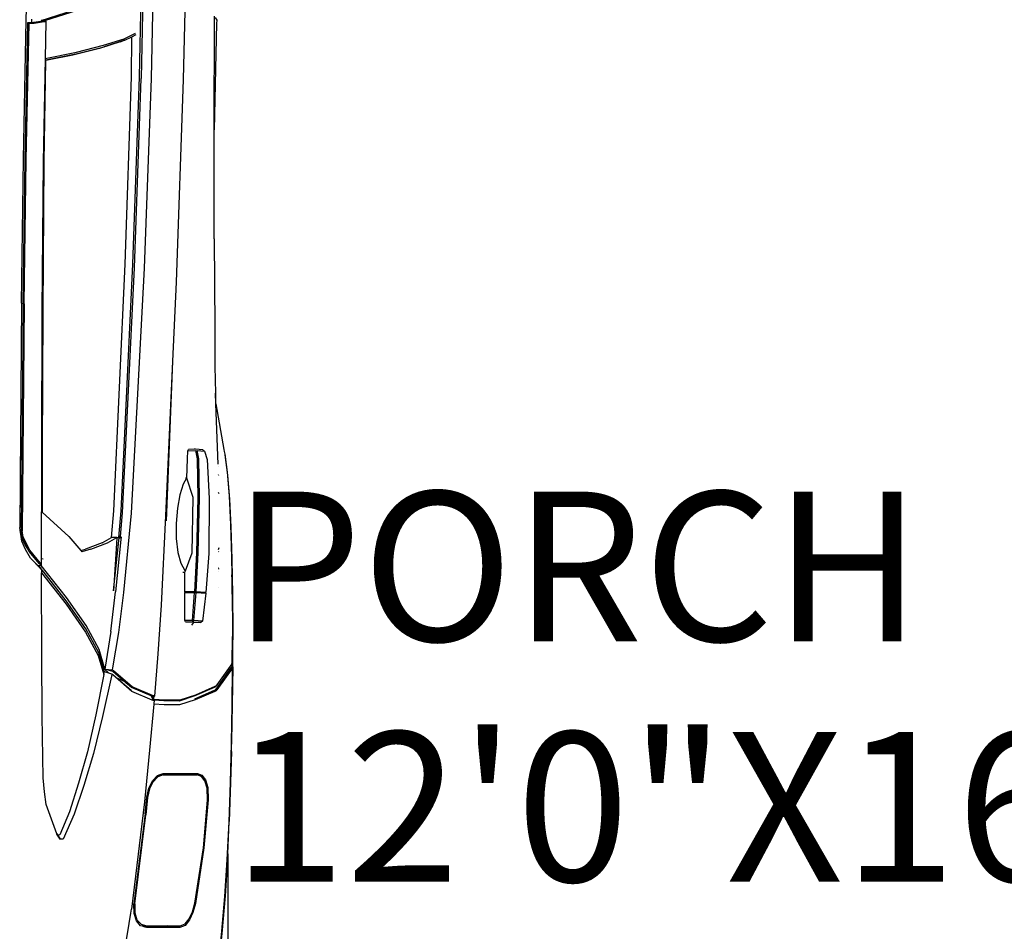
# Model space of a CAD drawing. Units: inches. Extents: x 22042254 to 25404563, y 17568978 to 17626777.
# Tile 30 of 45: x 22179876 to 22179932, y 17626227 to 17626279. Entities that reach past the tile are written whole.
import ezdxf

# ---------------------------------------------------------------- set-up
doc = ezdxf.new("R2010")
doc.units = ezdxf.units.IN
doc.header["$MEASUREMENT"] = 0
doc.layers.add('A-AREA-IDEN', color=7, linetype='Continuous', lineweight=18)
doc.layers.add('A-SITE-VEHI', color=8, linetype='Continuous', lineweight=18)
doc.layers.add('Edges', color=250, linetype='Continuous')
doc.styles.get("Standard").update_dxf_attribs({"font": 'arial.ttf'})

# ---------------------------------------------------------------- blocks, each defined once
blk = doc.blocks.new('Nissan Qashqai pl')
at = {"layer": 'Edges'}
for p, q in [((10.4304, 12.8056), (10.4339, 12.8061)), ((10.4339, 12.8061), (10.4573, 12.8093)), ((10.4339, 12.8061), (10.4345, 12.8062)), ((10.4345, 12.8062), (10.4613, 12.8099)), ((10.4573, 12.8093), (10.4889, 12.8119)), ((10.4613, 12.8099), (10.4926, 12.8125)), ((10.4889, 12.8119), (10.526, 12.8138)), ((10.4926, 12.8125), (10.5294, 12.8143)), ((10.526, 12.8138), (10.569, 12.8151)), ((10.5294, 12.8143), (10.5719, 12.8156)), ((10.569, 12.8151), (10.5919, 12.8155)), ((10.5719, 12.8156), (10.6176, 12.8164)), ((10.5919, 12.8155), (10.6151, 12.8159)), ((10.5981, 12.8157), (10.5919, 12.8155)), ((10.6174, 12.816), (10.5981, 12.8157)), ((10.6151, 12.8159), (10.6644, 12.8162)), ((10.6176, 12.8164), (10.6651, 12.8167)), ((10.6644, 12.8162), (10.7078, 12.8159)), ((10.6651, 12.8167), (10.666, 12.8167)), ((10.666, 12.8167), (10.677, 12.8167)), ((10.6729, 12.8157), (10.7082, 12.8156)), ((10.6809, 12.8167), (10.677, 12.8167)), ((10.7128, 12.8166), (10.6809, 12.8167)), ((10.7078, 12.8159), (10.7083, 12.8156)), ((10.7082, 12.8156), (10.7078, 12.8159)), ((10.7085, 12.8153), (10.7082, 12.8156)), ((10.7082, 12.8156), (10.7083, 12.8156)), ((10.7083, 12.8156), (10.7087, 12.8153)), ((10.7083, 12.8156), (10.7125, 12.8156)), ((10.7087, 12.8153), (10.7363, 12.7959)), ((10.7139, 12.8164), (10.7125, 12.8156)), ((10.7137, 12.8148), (10.7125, 12.8156)), ((10.7128, 12.8166), (10.7625, 12.8161)), ((10.7128, 12.8166), (10.724, 12.8166)), ((10.7137, 12.8148), (10.7138, 12.8147)), ((10.7418, 12.7947), (10.7138, 12.8147)), ((10.7139, 12.8164), (10.7148, 12.8157)), ((10.7628, 12.8158), (10.7139, 12.8164)), ((10.7148, 12.8157), (10.7429, 12.7956)), ((10.7685, 12.8161), (10.724, 12.8166)), ((10.7625, 12.8161), (10.7628, 12.8161)), ((10.7628, 12.8161), (10.8099, 12.8152)), ((10.8131, 12.8149), (10.7628, 12.8158)), ((10.7688, 12.8161), (10.7685, 12.8161)), ((10.8099, 12.8152), (10.7688, 12.8161)), ((10.8099, 12.8152), (10.8131, 12.8152)), ((10.8134, 12.8152), (10.8131, 12.8152)), ((10.8644, 12.8135), (10.8131, 12.8149)), ((10.8134, 12.8152), (10.8142, 12.8152)), ((10.8142, 12.8152), (10.8142, 12.8152)), ((10.8237, 12.8149), (10.8142, 12.8152)), ((10.8237, 12.8149), (10.864, 12.8138)), ((10.8596, 12.8138), (10.8589, 12.8138)), ((10.8642, 12.8136), (10.8596, 12.8138)), ((10.864, 12.8138), (10.8642, 12.8138)), ((10.8642, 12.8138), (10.9152, 12.812)), ((10.9158, 12.8118), (10.8644, 12.8135)), ((10.9577, 12.8101), (10.9152, 12.812)), ((10.9657, 12.8095), (10.9158, 12.8118)), ((10.9577, 12.8101), (10.9649, 12.8097)), ((10.9577, 12.8101), (11.1283, 12.8101)), ((10.9649, 12.8097), (11.0127, 12.8067)), ((11.0138, 12.8064), (10.9657, 12.8095)), ((11.0127, 12.8067), (11.0576, 12.8026)), ((11.059, 12.8023), (11.0138, 12.8064)), ((9.8614, 12.7937), (9.8647, 12.7956)), ((9.8647, 12.7956), (9.869, 12.7954)), ((9.869, 12.7954), (10.0085, 12.7922)), ((10.3189, 12.7931), (10.3537, 12.7939)), ((10.3537, 12.7939), (10.3832, 12.7945)), ((10.3679, 12.7944), (10.3537, 12.7939)), ((10.3679, 12.7944), (10.4275, 12.8051)), ((10.4468, 12.7976), (10.3679, 12.7944)), ((10.4275, 12.8051), (10.4304, 12.8056)), ((10.4503, 12.7976), (10.4502, 12.7976)), ((10.4603, 12.7976), (10.4613, 12.7978)), ((10.4838, 12.7977), (10.4852, 12.7982)), ((10.5565, 12.7985), (10.5591, 12.7977)), ((10.5615, 12.7978), (10.5617, 12.7985)), ((10.583, 12.7984), (10.5834, 12.798)), ((10.5836, 12.798), (10.5831, 12.7984)), ((10.5847, 12.798), (10.5841, 12.7984)), ((10.5873, 12.7981), (10.5873, 12.7981)), ((10.6087, 12.7983), (10.6087, 12.7984)), ((10.7363, 12.7959), (10.7376, 12.795)), ((10.7387, 12.794), (10.7376, 12.795)), ((10.7376, 12.795), (10.7378, 12.7946)), ((10.7378, 12.7946), (10.7379, 12.7945)), ((10.7378, 12.7946), (10.7385, 12.7932)), ((10.7385, 12.7932), (10.7497, 12.7679)), ((10.7387, 12.794), (10.7396, 12.7922)), ((10.743, 12.7939), (10.7418, 12.7947)), ((10.7432, 12.7954), (10.7426, 12.7954)), ((10.7429, 12.7956), (10.7432, 12.7954)), ((10.7434, 12.793), (10.743, 12.7939)), ((10.7441, 12.7954), (10.7432, 12.7954)), ((10.7432, 12.7954), (10.744, 12.7948)), ((10.744, 12.7948), (10.7448, 12.793)), ((11.0576, 12.8026), (11.0798, 12.8008)), ((11.0768, 12.8008), (11.059, 12.8023)), ((9.8643, 12.7927), (9.8598, 12.7928)), ((10.0085, 12.7922), (9.8643, 12.7927)), ((10.0124, 12.7922), (10.0085, 12.7922)), ((10.1513, 12.7924), (10.0124, 12.7922)), ((10.1513, 12.7924), (10.2677, 12.793)), ((10.2677, 12.793), (10.3189, 12.7931)), ((10.4299, 12.7798), (10.4406, 12.7829)), ((10.4406, 12.7829), (10.4919, 12.7858)), ((10.4919, 12.7858), (10.564, 12.7851)), ((10.564, 12.7851), (10.6151, 12.7813)), ((10.615, 12.7803), (10.6142, 12.7686)), ((10.6151, 12.7813), (10.615, 12.7803)), ((10.615, 12.7676), (10.6151, 12.7803)), ((10.6151, 12.7803), (10.615, 12.7803)), ((10.6151, 12.7803), (10.6151, 12.7813)), ((10.6151, 12.7685), (10.616, 12.7812)), ((10.616, 12.7812), (10.6526, 12.7768)), ((10.7396, 12.7922), (10.7507, 12.7669)), ((10.7437, 12.7921), (10.7434, 12.793)), ((10.7438, 12.7921), (10.7437, 12.7921)), ((10.7438, 12.7921), (10.7549, 12.7666)), ((10.7448, 12.793), (10.7559, 12.7674)), ((10.8546, 12.7762), (10.8607, 12.7808)), ((10.8607, 12.7808), (10.8708, 12.7841)), ((10.8716, 12.7832), (10.8622, 12.7801)), ((10.8708, 12.7841), (10.8869, 12.7844)), ((10.887, 12.7835), (10.8716, 12.7832)), ((10.8869, 12.7844), (10.9499, 12.7789)), ((10.9498, 12.7781), (10.887, 12.7835)), ((10.4263, 12.7665), (10.4274, 12.7674)), ((10.4282, 12.7775), (10.4274, 12.7679)), ((10.4274, 12.7679), (10.4274, 12.7674)), ((10.4274, 12.7674), (10.4275, 12.7586)), ((10.4282, 12.7775), (10.4299, 12.7798)), ((10.4291, 12.77), (10.4299, 12.7798)), ((10.4398, 12.7724), (10.4291, 12.77)), ((10.4291, 12.7677), (10.4398, 12.7701)), ((10.4293, 12.7579), (10.4291, 12.7677)), ((10.4909, 12.773), (10.4398, 12.7724)), ((10.4398, 12.7701), (10.4909, 12.7708)), ((10.5631, 12.7715), (10.4909, 12.773)), ((10.4909, 12.7708), (10.563, 12.7692)), ((10.563, 12.7692), (10.6142, 12.7663)), ((10.6142, 12.7686), (10.5631, 12.7715)), ((10.6142, 12.7686), (10.6142, 12.7677)), ((10.6142, 12.7677), (10.615, 12.7676)), ((10.6142, 12.7677), (10.6142, 12.7663)), ((10.6151, 12.7676), (10.615, 12.7676)), ((10.6518, 12.7657), (10.6151, 12.7685)), ((10.6151, 12.7676), (10.6151, 12.7685)), ((10.6151, 12.7662), (10.6151, 12.7676)), ((10.6526, 12.7768), (10.6518, 12.7657)), ((10.6526, 12.7768), (10.6543, 12.7749)), ((10.6537, 12.7658), (10.6543, 12.7749)), ((10.6543, 12.7749), (10.6543, 12.7656)), ((10.7497, 12.7679), (10.7565, 12.7473)), ((10.7559, 12.7674), (10.7626, 12.7467)), ((10.8523, 12.7704), (10.8546, 12.7762)), ((10.8523, 12.7255), (10.8523, 12.7704)), ((10.8543, 12.7702), (10.8538, 12.753)), ((10.8565, 12.7757), (10.8543, 12.7702)), ((10.8543, 12.7255), (10.8543, 12.7702)), ((10.8622, 12.7801), (10.8565, 12.7757)), ((11.0226, 12.7668), (10.9498, 12.7781)), ((10.9499, 12.7789), (11.0229, 12.7676)), ((11.0229, 12.7676), (11.0348, 12.7645)), ((9.8024, 12.7549), (9.9426, 12.7518)), ((10.4293, 12.7579), (10.4275, 12.7586)), ((10.4398, 12.7573), (10.4293, 12.7579)), ((10.4653, 12.7564), (10.4398, 12.7573)), ((10.4653, 12.7561), (10.4652, 12.7545)), ((10.4908, 12.7648), (10.4653, 12.7564)), ((10.4653, 12.7564), (10.4653, 12.7561)), ((10.4653, 12.7564), (10.4653, 12.7564)), ((10.4653, 12.7564), (10.4653, 12.7561)), ((10.4653, 12.7561), (10.4653, 12.7561)), ((10.4653, 12.7561), (10.4732, 12.7517)), ((10.563, 12.7633), (10.4908, 12.7648)), ((10.5867, 12.7545), (10.563, 12.7633)), ((10.5863, 12.7537), (10.5867, 12.7545)), ((10.5885, 12.7538), (10.5867, 12.7545)), ((10.6142, 12.766), (10.6141, 12.7537)), ((10.6142, 12.7663), (10.6142, 12.766)), ((10.615, 12.7537), (10.6151, 12.7659)), ((10.6151, 12.7662), (10.6518, 12.7634)), ((10.6151, 12.7659), (10.6151, 12.7662)), ((10.6518, 12.7634), (10.6517, 12.754)), ((10.6535, 12.7546), (10.6517, 12.754)), ((10.6536, 12.7639), (10.6518, 12.7657)), ((10.6518, 12.7657), (10.6518, 12.7634)), ((10.6518, 12.7634), (10.6536, 12.7639)), ((10.6543, 12.7656), (10.6535, 12.7546)), ((10.6535, 12.7546), (10.6536, 12.7639)), ((10.6536, 12.7639), (10.6537, 12.7658)), ((10.6537, 12.7658), (10.6543, 12.7656)), ((10.6578, 12.7628), (10.6543, 12.7656)), ((10.7507, 12.7669), (10.7575, 12.7462)), ((11.0339, 12.7639), (11.0226, 12.7668)), ((11.0429, 12.7597), (11.0339, 12.7639)), ((11.0348, 12.7645), (11.0444, 12.7601)), ((11.0497, 12.7542), (11.0429, 12.7597)), ((11.0444, 12.7601), (11.0516, 12.7542)), ((9.9426, 12.7518), (10.2081, 12.7424)), ((10.2081, 12.7424), (10.312, 12.7377)), ((10.4732, 12.7517), (10.4871, 12.7474)), ((10.4871, 12.7474), (10.5048, 12.744)), ((10.5048, 12.744), (10.5246, 12.7423)), ((10.5246, 12.7423), (10.5445, 12.7425)), ((10.5445, 12.7425), (10.5625, 12.7446)), ((10.5625, 12.7446), (10.5769, 12.7484)), ((10.5769, 12.7484), (10.5863, 12.7537)), ((10.5885, 12.751), (10.5885, 12.7538)), ((10.6141, 12.7537), (10.5885, 12.7538)), ((10.6141, 12.7537), (10.615, 12.7537)), ((10.6517, 12.754), (10.615, 12.7537)), ((10.7565, 12.7473), (10.7563, 12.7273)), ((10.7575, 12.7462), (10.7572, 12.7263)), ((10.7626, 12.7467), (10.7623, 12.7269)), ((10.8528, 12.7503), (10.8535, 12.7521)), ((10.8528, 12.742), (10.8528, 12.7503)), ((10.8528, 12.742), (10.8538, 12.742)), ((10.8528, 12.7419), (10.8528, 12.742)), ((10.8538, 12.7419), (10.8528, 12.7419)), ((10.8528, 12.7242), (10.8528, 12.7419)), ((10.8535, 12.7521), (10.8538, 12.753)), ((10.8538, 12.7521), (10.8535, 12.7521)), ((10.8538, 12.753), (10.8538, 12.7521)), ((10.8538, 12.7521), (10.8538, 12.7502)), ((10.8538, 12.7502), (10.8538, 12.742)), ((10.8538, 12.742), (10.8538, 12.7419)), ((10.8538, 12.7214), (10.8538, 12.7419)), ((11.0523, 12.7475), (11.0497, 12.7542)), ((11.0516, 12.7542), (11.0543, 12.7473)), ((11.0528, 12.73), (11.0523, 12.7475)), ((11.0523, 12.7312), (11.0523, 12.7475)), ((11.0543, 12.7473), (11.0543, 12.7035)), ((10.312, 12.7377), (10.5214, 12.7293)), ((10.312, 12.7377), (10.5147, 12.7285)), ((11.0523, 12.7312), (11.0528, 12.73)), ((11.0523, 12.7287), (11.0523, 12.7312)), ((11.0528, 12.7274), (11.0523, 12.7287)), ((11.0523, 12.7037), (11.0523, 12.7287)), ((11.0528, 12.7274), (11.0528, 12.73)), ((11.0528, 12.73), (11.0538, 12.7273)), ((10.5147, 12.7285), (10.6318, 12.7228)), ((10.6318, 12.7228), (10.6955, 12.7184)), ((10.6955, 12.7184), (10.7509, 12.714)), ((10.7563, 12.7273), (10.7553, 12.7134)), ((10.7572, 12.7263), (10.7563, 12.7126)), ((10.7623, 12.7269), (10.7615, 12.7131)), ((10.8528, 12.7242), (10.8523, 12.7255)), ((10.8538, 12.7214), (10.8528, 12.7242)), ((10.855, 12.7181), (10.8538, 12.7214)), ((10.8543, 12.7255), (10.8569, 12.7184)), ((10.8622, 12.7114), (10.855, 12.7181)), ((10.8569, 12.7184), (10.8637, 12.712)), ((11.0528, 12.7274), (11.0528, 12.6985)), ((11.0538, 12.7273), (11.0538, 12.7018)), ((9.9414, 12.71), (9.8143, 12.713)), ((10.19, 12.7008), (9.9414, 12.71)), ((10.7501, 12.7114), (10.7387, 12.6849)), ((10.7507, 12.7098), (10.7397, 12.684)), ((10.7563, 12.7109), (10.7449, 12.6843)), ((10.7507, 12.7132), (10.7501, 12.7114)), ((10.7506, 12.7111), (10.7507, 12.7132)), ((10.7507, 12.7132), (10.7509, 12.714)), ((10.751, 12.7132), (10.7507, 12.7132)), ((10.7511, 12.7107), (10.7507, 12.7098)), ((10.7524, 12.7106), (10.7507, 12.7098)), ((10.7522, 12.7131), (10.7509, 12.714)), ((10.7516, 12.7131), (10.7509, 12.714)), ((10.7519, 12.7128), (10.7511, 12.7107)), ((10.7522, 12.7131), (10.7516, 12.7131)), ((10.7519, 12.7128), (10.7516, 12.7131)), ((10.7526, 12.7124), (10.7519, 12.7128)), ((10.7553, 12.7134), (10.7522, 12.7131)), ((10.7524, 12.7106), (10.7526, 12.7124)), ((10.7556, 12.7122), (10.7524, 12.7106)), ((10.7526, 12.7124), (10.7526, 12.7127)), ((10.7532, 12.712), (10.7526, 12.7124)), ((10.7556, 12.7122), (10.7532, 12.712)), ((10.7561, 12.7125), (10.7556, 12.7122)), ((10.7561, 12.7125), (10.7563, 12.7126)), ((10.7563, 12.7125), (10.7561, 12.7125)), ((10.7563, 12.7123), (10.7561, 12.7123)), ((10.7563, 12.7126), (10.7573, 12.7135)), ((10.7563, 12.7126), (10.7563, 12.7125)), ((10.7569, 12.7125), (10.7563, 12.7109)), ((10.7569, 12.7125), (10.7563, 12.7125)), ((10.7563, 12.7125), (10.7563, 12.7123)), ((10.7573, 12.7135), (10.7569, 12.7125)), ((10.7573, 12.7135), (10.7604, 12.7132)), ((10.7604, 12.7132), (10.7615, 12.7131)), ((10.7615, 12.7131), (10.8218, 12.7077)), ((10.8218, 12.7077), (10.8896, 12.7008)), ((10.8718, 12.7068), (10.8622, 12.7114)), ((10.8637, 12.712), (10.8727, 12.7077)), ((10.8836, 12.7041), (10.8718, 12.7068)), ((10.8727, 12.7077), (10.8839, 12.7051)), ((10.9054, 12.702), (10.8836, 12.7041)), ((10.8839, 12.7051), (10.9067, 12.7029)), ((11.0231, 12.6882), (10.9067, 12.7029)), ((11.0501, 12.6964), (11.0523, 12.7037)), ((11.0543, 12.7035), (11.0538, 12.7018)), ((9.8101, 12.6993), (9.9411, 12.6966)), ((9.9393, 12.6944), (9.8119, 12.697)), ((9.8867, 12.6842), (9.8838, 12.6901)), ((10.1849, 12.6857), (9.9393, 12.6944)), ((10.1894, 12.6879), (9.9411, 12.6966)), ((10.5113, 12.6839), (10.19, 12.7008)), ((10.8896, 12.7008), (11.0304, 12.6838)), ((10.9054, 12.702), (11.0232, 12.6871)), ((11.035, 12.6883), (11.0443, 12.6911)), ((11.0458, 12.6903), (11.0358, 12.6872)), ((11.0443, 12.6911), (11.0501, 12.6964)), ((11.052, 12.6958), (11.0458, 12.6903)), ((11.0528, 12.6985), (11.052, 12.6958)), ((11.0538, 12.7018), (11.0528, 12.6985)), ((9.8891, 12.6741), (9.8818, 12.6891)), ((9.9393, 12.684), (9.8867, 12.6842)), ((9.8911, 12.675), (9.8867, 12.6842)), ((10.1849, 12.6754), (9.9393, 12.684)), ((10.5079, 12.6703), (10.1849, 12.6857)), ((10.5109, 12.6721), (10.1894, 12.6879)), ((10.6152, 12.674), (10.5113, 12.6839)), ((10.7387, 12.6849), (10.7177, 12.6604)), ((10.7449, 12.6843), (10.7232, 12.6594)), ((10.7438, 12.6836), (10.7265, 12.6635)), ((10.7397, 12.684), (10.7334, 12.6766)), ((11.0231, 12.6882), (11.035, 12.6883)), ((11.0358, 12.6872), (11.0232, 12.6871)), ((11.0357, 12.6829), (11.0304, 12.6838)), ((11.0491, 12.6807), (11.0357, 12.6829)), ((11.0449, 12.6812), (11.0448, 12.6812)), ((11.0492, 12.6807), (11.0491, 12.6807)), ((11.1336, 12.667), (11.0492, 12.6807)), ((9.8978, 12.6472), (9.8891, 12.6741)), ((9.8911, 12.6749), (9.8911, 12.675)), ((9.8931, 12.6691), (9.8911, 12.6749)), ((9.8911, 12.6749), (9.8998, 12.6481)), ((9.8931, 12.669), (9.8931, 12.6691)), ((9.8931, 12.669), (9.9018, 12.6421)), ((10.5079, 12.6607), (10.1849, 12.6754)), ((10.543, 12.6671), (10.5079, 12.6703)), ((10.5417, 12.6693), (10.5109, 12.6721)), ((10.5417, 12.6693), (10.5427, 12.6702)), ((10.5417, 12.6693), (10.543, 12.6671)), ((10.5436, 12.6687), (10.5427, 12.6702)), ((10.5427, 12.6702), (10.5458, 12.67)), ((10.544, 12.6678), (10.543, 12.6671)), ((10.543, 12.6646), (10.543, 12.6671)), ((10.543, 12.6646), (10.543, 12.6576)), ((10.5439, 12.6646), (10.543, 12.6646)), ((10.5502, 12.6526), (10.543, 12.6646)), ((10.544, 12.6678), (10.5436, 12.6687)), ((10.5439, 12.6646), (10.613, 12.6601)), ((10.547, 12.6674), (10.544, 12.6678)), ((10.5458, 12.67), (10.6144, 12.6629)), ((10.613, 12.6601), (10.547, 12.6674)), ((10.6678, 12.6672), (10.6152, 12.674)), ((10.7137, 12.6595), (10.6678, 12.6672)), ((10.7334, 12.6766), (10.7186, 12.6593)), ((10.7265, 12.6635), (10.7316, 12.6741)), ((10.543, 12.6576), (10.5079, 12.6607)), ((10.5502, 12.6456), (10.543, 12.6576)), ((10.5584, 12.6306), (10.5502, 12.6526)), ((10.6664, 12.6566), (10.6144, 12.6629)), ((10.6664, 12.6566), (10.7155, 12.649)), ((10.7165, 12.6591), (10.7137, 12.6595)), ((10.7186, 12.6593), (10.7155, 12.649)), ((10.7155, 12.649), (10.7165, 12.6591)), ((10.7209, 12.654), (10.7155, 12.6485)), ((10.7177, 12.6604), (10.7165, 12.6591)), ((10.7209, 12.654), (10.7192, 12.6484)), ((10.7221, 12.6581), (10.7209, 12.654)), ((10.7232, 12.6594), (10.7221, 12.6581)), ((10.7221, 12.6581), (10.7224, 12.6587)), ((10.7221, 12.6581), (10.7247, 12.6575)), ((10.7265, 12.6635), (10.7224, 12.6587)), ((10.7247, 12.6575), (10.7776, 12.646)), ((9.9066, 12.6119), (9.8978, 12.6472)), ((9.9086, 12.6129), (9.8998, 12.6481)), ((9.9018, 12.6421), (9.9106, 12.6068)), ((10.5502, 12.6456), (10.5584, 12.6236)), ((10.69, 12.6414), (10.6583, 12.6245)), ((10.6943, 12.641), (10.6627, 12.6241)), ((10.6671, 12.6238), (10.6976, 12.6401)), ((10.7155, 12.649), (10.69, 12.6414)), ((10.7155, 12.6473), (10.6943, 12.641)), ((10.6976, 12.6401), (10.7228, 12.6477)), ((10.7155, 12.649), (10.7155, 12.6485)), ((10.7155, 12.6485), (10.7155, 12.6473)), ((10.7192, 12.6484), (10.7155, 12.6473)), ((10.7228, 12.6477), (10.7192, 12.6484)), ((10.7228, 12.6477), (10.7754, 12.637)), ((10.7776, 12.646), (10.8264, 12.6341)), ((10.5584, 12.6306), (10.5617, 12.619)), ((10.7754, 12.637), (10.8239, 12.6261)), ((10.8239, 12.6261), (10.8653, 12.6144)), ((10.8264, 12.6341), (10.8682, 12.6216)), ((9.8652, 12.5704), (9.8516, 12.6129)), ((9.9169, 12.5714), (9.9086, 12.6129)), ((10.5419, 12.6018), (10.56, 12.6176)), ((10.56, 12.6176), (10.5584, 12.6236)), ((10.56, 12.6176), (10.5617, 12.619)), ((10.6583, 12.6245), (10.6215, 12.5986)), ((10.6627, 12.6241), (10.6261, 12.5984)), ((10.6306, 12.5982), (10.6671, 12.6238)), ((10.8653, 12.6144), (10.9026, 12.6025)), ((10.8682, 12.6216), (10.9059, 12.6087)), ((9.8652, 12.5654), (9.8516, 12.6079)), ((9.9149, 12.5705), (9.9066, 12.6119)), ((9.9106, 12.6068), (9.9177, 12.5714)), ((10.51, 12.5666), (10.5419, 12.6018)), ((10.9026, 12.6025), (10.933, 12.5901)), ((10.9059, 12.6087), (10.9384, 12.5945)), ((10.6215, 12.5986), (10.5796, 12.5655)), ((10.5892, 12.5659), (10.6306, 12.5982)), ((10.6261, 12.5984), (10.593, 12.5726)), ((10.9316, 12.586), (10.9334, 12.5872)), ((10.9335, 12.5871), (10.932, 12.5862)), ((10.933, 12.5901), (10.9334, 12.5872)), ((10.9334, 12.5872), (10.9386, 12.5905)), ((10.9334, 12.5872), (10.9335, 12.5871)), ((10.9386, 12.5905), (10.9335, 12.5871)), ((10.9384, 12.5945), (10.9386, 12.5905)), ((10.9316, 12.586), (10.8932, 12.572)), ((10.932, 12.5862), (10.9316, 12.586)), ((9.8652, 12.5706), (9.8664, 12.5714)), ((9.8652, 12.5706), (9.8665, 12.5695)), ((9.8652, 12.5704), (9.8652, 12.5706)), ((9.8652, 12.5704), (9.8652, 12.5704)), ((9.8652, 12.5704), (9.8652, 12.5654)), ((9.8655, 12.5687), (9.8652, 12.5704)), ((9.8675, 12.5555), (9.8655, 12.5687)), ((9.8665, 12.5695), (9.8664, 12.5714)), ((9.8664, 12.5714), (9.9149, 12.5705)), ((9.8686, 12.5562), (9.8665, 12.5695)), ((9.9149, 12.5705), (10.0505, 12.5681)), ((9.9177, 12.5714), (9.9169, 12.5714)), ((10.0501, 12.5695), (9.9177, 12.5714)), ((10.2453, 12.568), (10.0501, 12.5695)), ((10.0505, 12.5681), (10.2453, 12.5664)), ((10.4292, 12.5674), (10.2453, 12.568)), ((10.2453, 12.5664), (10.4289, 12.5658)), ((10.4289, 12.5658), (10.5092, 12.5658)), ((10.5099, 12.5674), (10.4292, 12.5674)), ((10.5099, 12.5674), (10.5092, 12.5658)), ((10.5092, 12.5658), (10.5094, 12.5658)), ((10.5094, 12.5658), (10.51, 12.5666)), ((10.5783, 12.5659), (10.5094, 12.5658)), ((10.51, 12.5666), (10.5099, 12.5674)), ((10.5764, 12.5642), (10.5598, 12.5507)), ((10.5776, 12.5633), (10.5612, 12.5498)), ((10.5834, 12.5641), (10.57, 12.5517)), ((10.57, 12.5517), (10.5821, 12.5633)), ((10.5709, 12.5675), (10.5705, 12.5671)), ((10.5719, 12.5682), (10.5709, 12.5675)), ((10.5783, 12.5659), (10.5764, 12.5642)), ((10.5776, 12.5633), (10.5783, 12.5659)), ((10.5796, 12.5655), (10.5776, 12.5633)), ((10.5796, 12.5655), (10.5783, 12.5659)), ((10.5796, 12.562), (10.5796, 12.5655)), ((10.5838, 12.5653), (10.5821, 12.5633)), ((10.584, 12.5647), (10.5834, 12.5641)), ((10.584, 12.5655), (10.5838, 12.5653)), ((10.593, 12.5726), (10.584, 12.5655)), ((10.584, 12.5655), (10.5841, 12.5655)), ((10.584, 12.5654), (10.584, 12.5655)), ((10.5847, 12.5655), (10.584, 12.5647)), ((10.584, 12.5647), (10.584, 12.5654)), ((10.5851, 12.5659), (10.5841, 12.5655)), ((10.5841, 12.5655), (10.5847, 12.5655)), ((10.5851, 12.5659), (10.5847, 12.5655)), ((10.5851, 12.5659), (10.5892, 12.5659)), ((10.6988, 12.5662), (10.5892, 12.5659)), ((10.7769, 12.5667), (10.6988, 12.5662)), ((10.858, 12.5683), (10.7769, 12.5667)), ((10.8766, 12.5697), (10.858, 12.5683)), ((10.8932, 12.572), (10.8766, 12.5697)), ((9.8644, 12.5459), (9.696, 12.551)), ((9.8643, 12.5532), (9.8637, 12.5532)), ((9.8677, 12.5531), (9.8643, 12.5532)), ((9.8677, 12.5531), (9.8675, 12.5555)), ((9.8678, 12.5507), (9.8677, 12.5531)), ((9.8681, 12.5482), (9.8678, 12.5507)), ((9.8681, 12.5482), (9.869, 12.5496)), ((10.0476, 12.5445), (9.8681, 12.5482)), ((9.8689, 12.5515), (9.8686, 12.5562)), ((9.869, 12.5496), (9.8689, 12.5515)), ((10.0477, 12.5459), (9.869, 12.5496)), ((10.5598, 12.5507), (10.5522, 12.5465)), ((10.5583, 12.5481), (10.5546, 12.546)), ((10.5551, 12.5457), (10.5583, 12.5481)), ((10.5612, 12.5498), (10.5583, 12.5481)), ((10.57, 12.5517), (10.5589, 12.5451)), ((10.0472, 12.5423), (9.8644, 12.5459)), ((10.2357, 12.5398), (10.0472, 12.5423)), ((10.2367, 12.5419), (10.0476, 12.5445)), ((10.2369, 12.5433), (10.0477, 12.5459)), ((10.2357, 12.5398), (10.53, 12.5373)), ((10.2367, 12.5419), (10.5351, 12.5392)), ((10.2369, 12.5433), (10.5348, 12.5406)), ((10.4153, 12.5384), (10.4176, 12.5384)), ((10.4176, 12.5384), (10.4181, 12.5384)), ((10.4181, 12.5384), (10.4552, 12.538)), ((10.4181, 12.5384), (10.4181, 12.5384)), ((10.4778, 12.5378), (10.53, 12.5373)), ((10.5301, 12.5373), (10.53, 12.5373)), ((10.5335, 12.5378), (10.5301, 12.5373)), ((10.5419, 12.5391), (10.5335, 12.5378)), ((10.5422, 12.542), (10.5348, 12.5406)), ((10.5418, 12.5405), (10.5351, 12.5392)), ((10.5424, 12.5406), (10.5418, 12.5405)), ((10.5419, 12.5391), (10.5463, 12.541)), ((10.5479, 12.54), (10.5419, 12.5391)), ((10.5522, 12.5465), (10.5422, 12.542)), ((10.5495, 12.5438), (10.5424, 12.5406)), ((10.5463, 12.541), (10.5551, 12.5457)), ((10.5589, 12.5451), (10.5479, 12.54)), ((10.5546, 12.546), (10.5495, 12.5438))]:
    blk.add_line(p, q, dxfattribs=at)
blk = doc.blocks.new('CAR')
blk.add_blockref('Nissan Qashqai pl', (-9.7433, -11.9151))

msp = doc.modelspace()

# ---------------------------------------------------------------- block references
at = {"layer": 'A-SITE-VEHI', "xscale": 43.56002006885659, "yscale": 43.56002006885659, "zscale": 43.56002006885659, "rotation": 270}
msp.add_blockref('CAR', (22179848.861, 17626284.325), dxfattribs=at)

# ---------------------------------------------------------------- texts
at = {"layer": 'A-AREA-IDEN'}
for s, height, p in [('PORCH', 8.5453, (22179888.134, 17626243.566)), ('12\'0"X16\'8"', 8.54529, (22179888.134, 17626229.838))]:
    msp.add_text(s, height=height, dxfattribs=at).set_placement(p)

doc.saveas('drawing.dxf')
